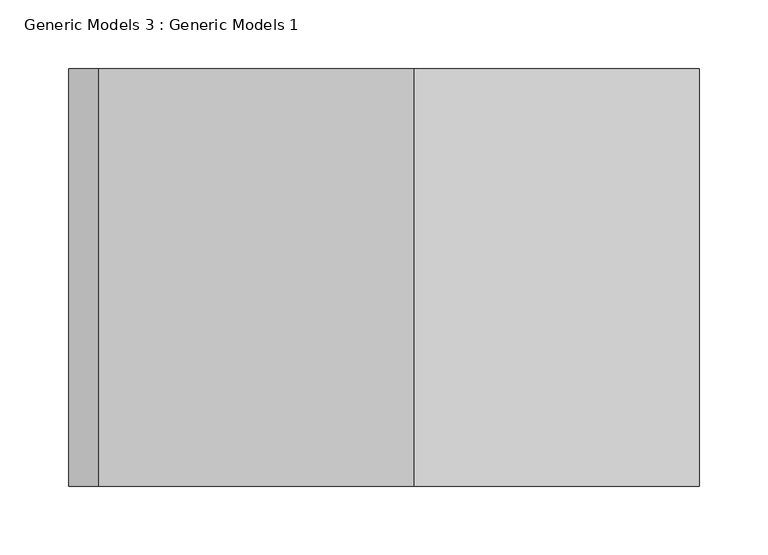
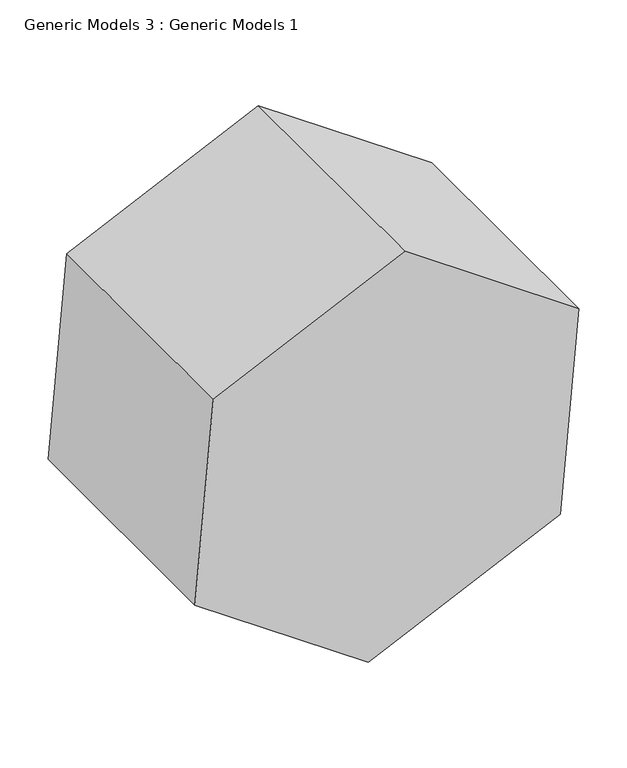
"""IFC4 building model written with IfcOpenShell, lengths in millimetres: proxy geometry, Generic Models 3 : Generic Models 1."""

from ifc_helpers import new_model, si_unit, frame, origin, place, context, project, spatial, polyline, outline, extrude, source, transform, mapped, element, save


def generic_models_3_generic_models_1_4242ebdf(model_context):
    return source(origin(), model_context, "Body", "SweptSolid", [
        extrude(outline(polyline([(833.1013393, -5439.1079055), (978.7897542, -5647.1725247), (871.4447157, -5877.3747026), (618.4112624, -5899.5122613), (472.7228475, -5691.447642), (580.067886, -5461.2454641), (833.1013393, -5439.1079055)])), frame((0.0, -10720.3372434, 0.0), z_axis=(0.0, 1.0, 0.0), x_axis=(0.0, 0.0, 1.0)), (0.0, 0.0, 1.0), 304.8),
    ])


if __name__ == "__main__":
    model = new_model("IFC4")
    model_context = context("Model", 3, world=origin())
    ifc_project = project(units=[si_unit("LENGTHUNIT", "METRE", prefix="MILLI")], contexts=[model_context])
    site = spatial("IfcSite", under=ifc_project)
    building = spatial("IfcBuilding", under=site)
    placement = place(None, origin())
    generic_models_3_generic_models_1_shape = generic_models_3_generic_models_1_4242ebdf(model_context)
    element("IfcBuildingElementProxy", 1, Name="Generic Models 3 : Generic Models 1", ObjectType="Generic Models 3 : Generic Models 1", at=placement, inside=building, context=model_context, shape_type="MappedRepresentation", body=[
        mapped(generic_models_3_generic_models_1_shape, transform((0.0, 0.0, 0.0), x_axis=(1.0, 0.0, 0.0), y_axis=(0.0, 1.0, 0.0), z_axis=(0.0, 0.0, 1.0))),
    ])
    save(model, "model.ifc")
